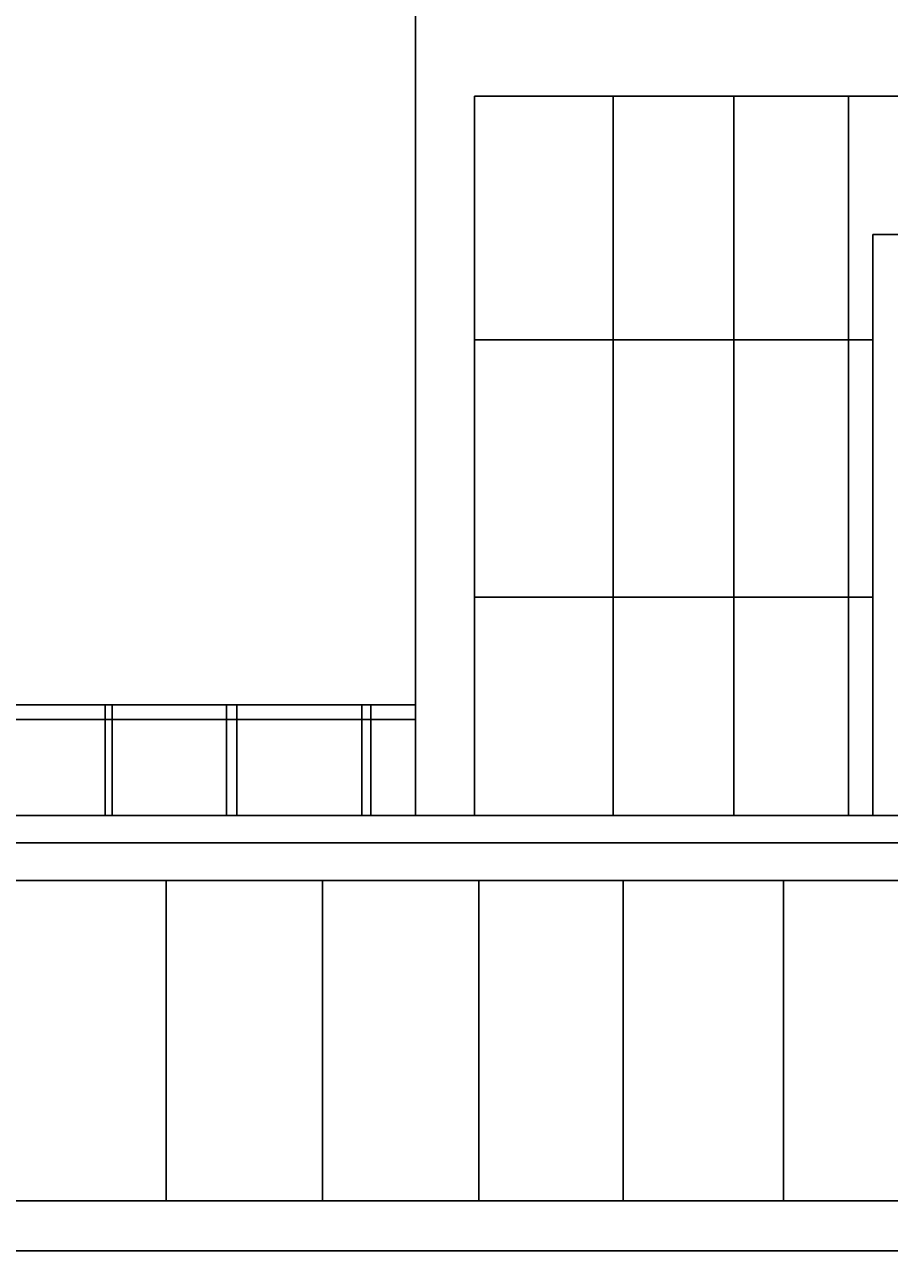
# Model space of a CAD drawing. Units: inches. Extents: x -117 to 121, y -77 to 40.
# Tile 12 of 45: x -85 to -64, y -23 to 7. Entities that reach past the tile are written whole.
import ezdxf

# ---------------------------------------------------------------- set-up
doc = ezdxf.new("R2010")
doc.units = ezdxf.units.IN
doc.header["$MEASUREMENT"] = 0
doc.layers.add('A-ANNO-DIMS', color=2, linetype='Continuous', lineweight=18)
doc.layers.add('A-ELEV', color=7, linetype='Continuous', lineweight=25)
doc.styles.get("Standard").update_dxf_attribs({"font": 'arial.ttf'})
doc.dimstyles.get("Standard").update_dxf_attribs({"dimtxt": 0.18, "dimasz": 0.18, "dimexe": 0.18, "dimexo": 0.0625, "dimgap": 0.09, "dimtad": 0, "dimtih": 1, "dimtoh": 1, "dimdec": 4, "dimzin": 0, "dimdsep": 46, "dimtxsty": 'Standard', "dimcen": 0.09, "dimadec": 0, "dimazin": 0, "dimtfac": 1, "dimtdec": 4, "dimtofl": 0, "dimtmove": 0, "dimatfit": 3, "dimfxl": 1, "dimtolj": 1, "dimtzin": 0, "dimarcsym": 0})

# ---------------------------------------------------------------- blocks, each defined once
blk = doc.blocks.new('*D13')
at = {"layer": 'A-ANNO-DIMS', "color": 0, "lineweight": -2, "transparency": 16777216}
for p, q in [((-2.663, 27.063), (-117.024, 27.063)), ((-116.844, 26.883), (-116.844, -16.974)), ((-116.844, -61.196), (-116.844, -17.338)), ((-106.096, -61.376), (-117.024, -61.376))]:
    blk.add_line(p, q, dxfattribs=at)
at = {"layer": 'A-ANNO-DIMS', "color": 0, "transparency": 16777216}
for points in [[(-116.874, 26.883), (-116.814, 26.883), (-116.844, 27.063)], [(-116.874, -61.196), (-116.814, -61.196), (-116.844, -61.376)]]:
    blk.add_solid(points, dxfattribs=at)
at = {"layer": 'Defpoints', "color": 0, "transparency": 16777216}
for p in [(-2.6, 27.063), (-116.844, -61.376), (-106.034, -61.376)]:
    blk.add_point(p, dxfattribs=at)
at = {"layer": 'A-ANNO-DIMS', "color": 0, "transparency": 16777216, "insert": (-116.844, -17.156), "char_height": 0.18, "attachment_point": 5}
blk.add_mtext('\\A1;88.44', dxfattribs=at)
blk = doc.blocks.new('*D20')
at = {"layer": 'A-ANNO-DIMS', "color": 0, "lineweight": -2, "transparency": 16777216}
for p, q in [((-75.866, 11.871), (-117.024, 11.871)), ((-116.844, 11.691), (-116.844, 0.051)), ((-116.844, -11.953), (-116.844, -0.313)), ((-94.498, -12.133), (-117.024, -12.133))]:
    blk.add_line(p, q, dxfattribs=at)
at = {"layer": 'A-ANNO-DIMS', "color": 0, "transparency": 16777216}
for points in [[(-116.874, 11.691), (-116.814, 11.691), (-116.844, 11.871)], [(-116.874, -11.953), (-116.814, -11.953), (-116.844, -12.133)]]:
    blk.add_solid(points, dxfattribs=at)
at = {"layer": 'Defpoints', "color": 0, "transparency": 16777216}
for p in [(-75.804, 11.871), (-116.844, -12.133), (-94.436, -12.133)]:
    blk.add_point(p, dxfattribs=at)
at = {"layer": 'A-ANNO-DIMS', "color": 0, "transparency": 16777216, "insert": (-116.844, -0.131), "char_height": 0.18, "attachment_point": 5}
blk.add_mtext('\\A1;24.004', dxfattribs=at)
blk = doc.blocks.new('*D21')
at = {"layer": 'A-ANNO-DIMS', "color": 0, "lineweight": -2, "transparency": 16777216}
for p, q in [((-106.034, -61.313), (-106.034, 38.61)), ((-75.804, 8.087), (-75.804, 38.61)), ((-105.854, 38.43), (-91.382, 38.43)), ((-75.984, 38.43), (-90.455, 38.43))]:
    blk.add_line(p, q, dxfattribs=at)
at = {"layer": 'A-ANNO-DIMS', "color": 0, "transparency": 16777216}
for points in [[(-105.854, 38.46), (-105.854, 38.4), (-106.034, 38.43)], [(-75.984, 38.46), (-75.984, 38.4), (-75.804, 38.43)]]:
    blk.add_solid(points, dxfattribs=at)
at = {"layer": 'Defpoints', "color": 0, "transparency": 16777216}
for p in [(-75.804, 38.43), (-75.804, 8.025), (-106.034, -61.376)]:
    blk.add_point(p, dxfattribs=at)
at = {"layer": 'A-ANNO-DIMS', "color": 0, "transparency": 16777216, "insert": (-90.919, 38.43), "char_height": 0.18, "attachment_point": 5}
blk.add_mtext('\\A1;30.230', dxfattribs=at)
blk = doc.blocks.new('*D40')
at = {"layer": 'A-ANNO-DIMS', "color": 0, "lineweight": -2, "transparency": 16777216}
for p, q in [((-86.023, -13.677), (-86.023, 38.61)), ((-63.159, -13.677), (-63.159, 38.61)), ((-85.843, 38.43), (-75.056, 38.43)), ((-63.339, 38.43), (-74.126, 38.43))]:
    blk.add_line(p, q, dxfattribs=at)
at = {"layer": 'A-ANNO-DIMS', "color": 0, "transparency": 16777216}
for points in [[(-85.843, 38.46), (-85.843, 38.4), (-86.023, 38.43)], [(-63.339, 38.46), (-63.339, 38.4), (-63.159, 38.43)]]:
    blk.add_solid(points, dxfattribs=at)
at = {"layer": 'Defpoints', "color": 0, "transparency": 16777216}
for p in [(-63.159, 38.43), (-86.023, -13.74), (-63.159, -13.74)]:
    blk.add_point(p, dxfattribs=at)
at = {"layer": 'A-ANNO-DIMS', "color": 0, "transparency": 16777216, "insert": (-74.591, 38.43), "char_height": 0.18, "attachment_point": 5}
blk.add_mtext('\\A1;22.864', dxfattribs=at)

msp = doc.modelspace()

# ---------------------------------------------------------------- linework, layer by layer
at = {"layer": 'A-ELEV'}
for p, q in [((-75.8037, 9.0994), (-75.8037, -3.0042)), ((-23.8637, 5.6231), (-74.3507, 5.6231)), ((-74.3507, -12.1334), (-74.3507, 5.6231)), ((-70.9247, -12.1334), (-70.9247, 5.6231)), ((-67.9455, -12.1334), (-67.9455, 5.6231)), ((-65.1153, -12.1334), (-65.1153, 5.6231)), ((-64.513, -9.5631), (-64.513, 2.2073)), ((-64.513, 2.2073), (-27.4892, 2.2073)), ((-74.3507, -0.3942), (-64.513, -0.3942)), ((-75.8037, -3.0042), (-75.8037, -12.1334)), ((-74.3507, -6.7428), (-64.513, -6.7428)), ((-94.4355, -9.4047), (-75.8037, -9.4047)), ((-83.4712, -12.1334), (-83.4712, -9.4047)), ((-83.2949, -12.1334), (-83.2949, -9.4047)), ((-80.4719, -12.1334), (-80.4719, -9.4047)), ((-80.221, -12.1334), (-80.221, -9.4047)), ((-77.1314, -12.1334), (-77.1314, -9.4047)), ((-76.9118, -12.1334), (-76.9118, -9.4047)), ((-94.4355, -9.7631), (-75.8037, -9.7631)), ((-64.513, -9.5631), (-64.513, -12.1334)), ((-64.513, -12.1334), (-94.4355, -12.1334)), ((-75.8037, -12.1334), (-74.3507, -12.1334)), ((-64.513, -12.1334), (-45.4848, -12.1334)), ((-64.513, -12.8131), (-93.028, -12.8131)), ((-64.513, -12.8131), (-46.5108, -12.8131)), ((-64.513, -13.74), (-86.0225, -13.74)), ((-81.9645, -21.6476), (-81.9645, -13.74)), ((-78.1044, -21.6476), (-78.1044, -13.74)), ((-74.2443, -21.6476), (-74.2443, -13.74)), ((-70.6811, -21.6476), (-70.6811, -13.74)), ((-66.7221, -21.6476), (-66.7221, -13.74)), ((-64.513, -13.74), (-62.763, -13.74)), ((-64.513, -21.6476), (-86.0225, -21.6476)), ((-64.513, -21.6476), (-62.763, -21.6476)), ((-46.5108, -22.8827), (-93.028, -22.8827))]:
    msp.add_line(p, q, dxfattribs=at)

# ---------------------------------------------------------------- dimensions: what is measured, and where the dimension line sits
at = {"layer": 'A-ANNO-DIMS'}
for base, p1, p2, picture, middle in [((-75.8037, 38.4297), (-106.0338, -61.3756), (-75.8037, 8.0246), '*D21', (-90.9187, 38.4297)), ((-63.1589, 38.4297), (-86.0225, -13.74), (-63.1589, -13.74), '*D40', (-74.5907, 38.4297))]:
    dim = msp.add_linear_dim(base=base, p1=p1, p2=p2, dimstyle='Standard', override={"dimdec": 3, "dimlfac": 1, "dimrnd": 0, "dimzin": 0, "dimdsep": 46, "dimlunit": 2}, dxfattribs=at)
    dim.commit()
    dim.dimension.update_dxf_attribs({"geometry": picture, "text_midpoint": middle})
for base, p1, p2, override, picture, middle in [((-116.8438, -61.3756), (-2.6001, 27.0634), (-106.0338, -61.3756), {"dimdec": 2, "dimlfac": 1, "dimrnd": 0, "dimzin": 0, "dimdsep": 46, "dimlunit": 2}, '*D13', (-116.8438, -17.1561)), ((-116.84377, -12.13336), (-75.80372, 11.87111), (-94.43553, -12.13336), {"dimdec": 3, "dimlfac": 1, "dimrnd": 0, "dimzin": 0, "dimdsep": 46, "dimlunit": 2}, '*D20', (-116.84377, -0.13113))]:
    dim = msp.add_linear_dim(base=base, p1=p1, p2=p2, angle=90, dimstyle='Standard', override=override, dxfattribs=at)
    dim.commit()
    dim.dimension.update_dxf_attribs({"geometry": picture, "text_midpoint": middle})

doc.saveas('drawing.dxf')
